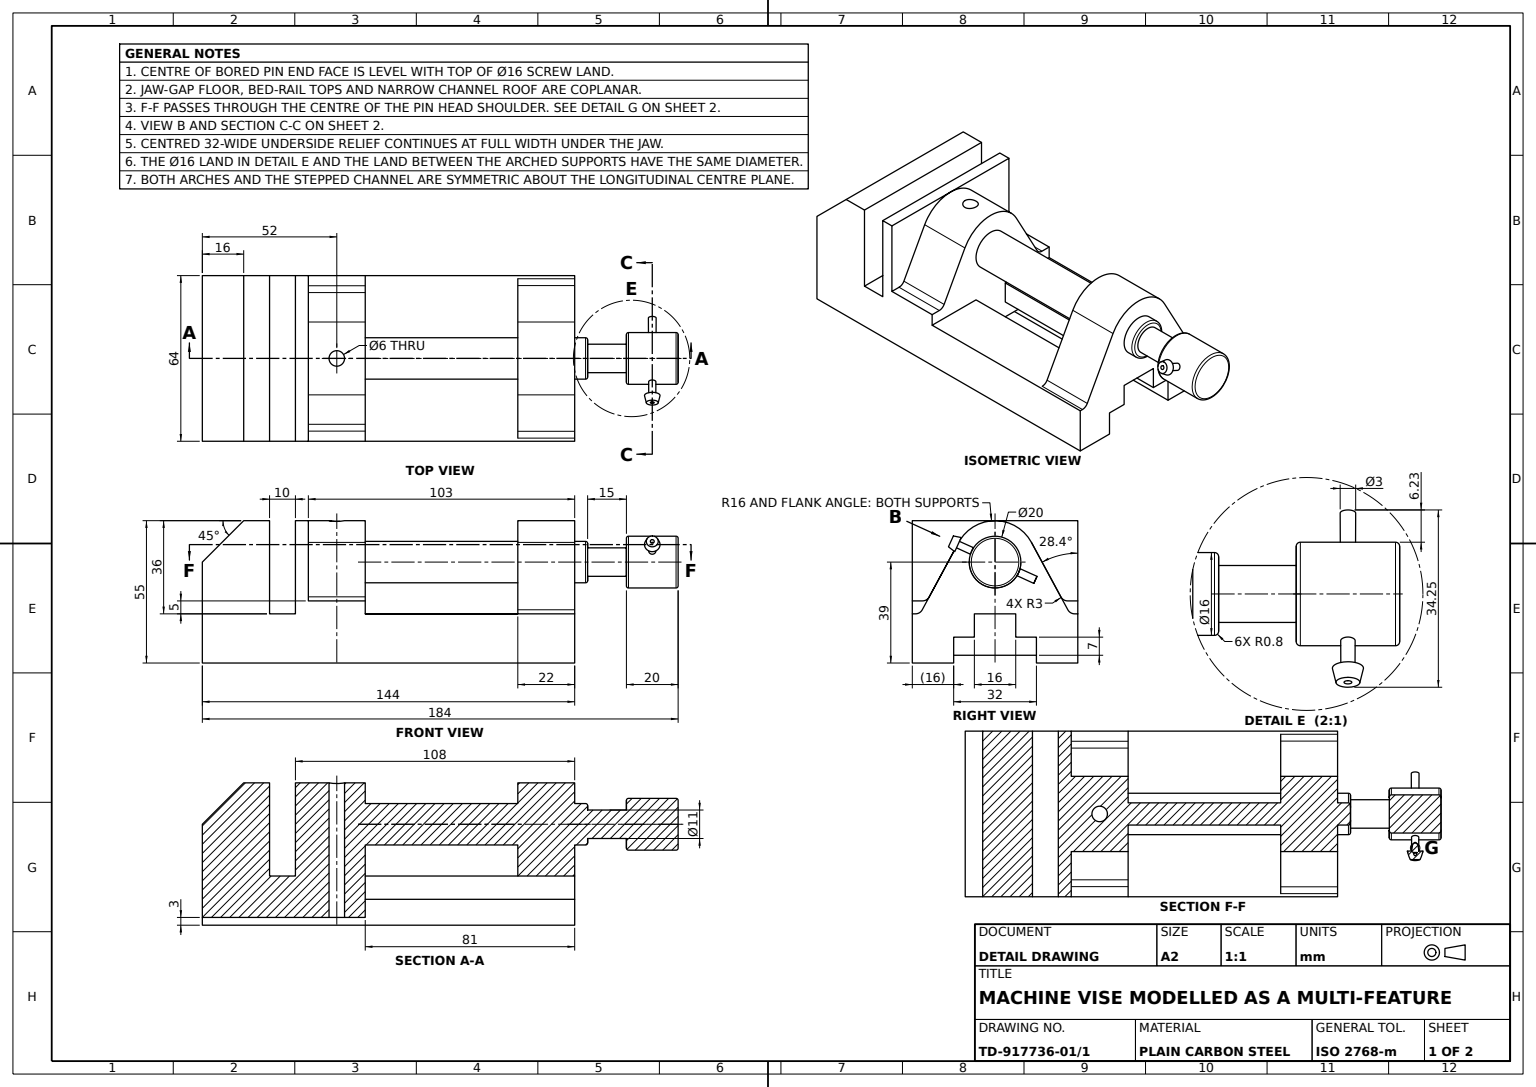
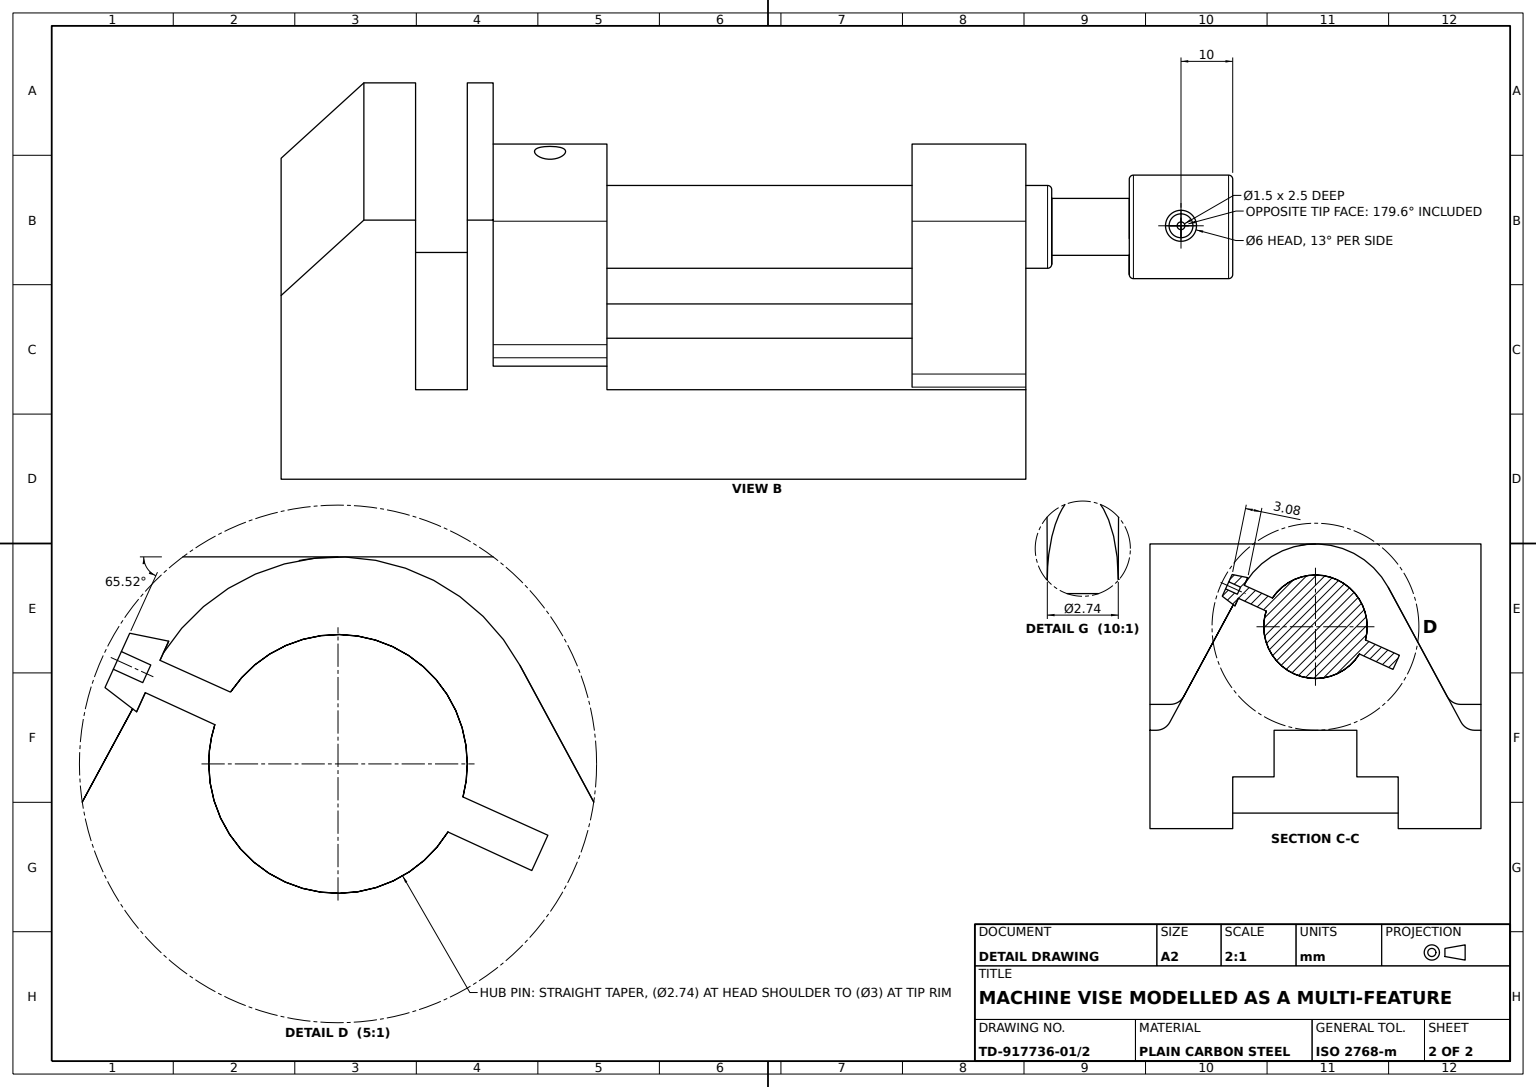
from build123d import *

# Parameters (mm, degrees)
VISE_BODY_DEPTH                 = 64
GUIDE_CHANNEL_PROFILE_OUTSIDE_W = 99.188
GUIDE_CHANNEL_PROFILE_OUTSIDE_H = 87.188
GUIDE_CHANNEL_CUT_DEPTH         = 81
SUPPORT_PLATE_PROFILE_W         = 64
SUPPORT_PLATE_PROFILE_H         = 52
SUPPORT_PLATE_DEPTH             = 5
JAW_START                       = 22
JAW_BLOCK_DEPTH                 = 22
LEAD_SCREW_SHAFT_16_DEPTH       = 5
LEAD_SCREW_SHAFT_16_DEPTH_BACK  = 81
LEAD_SCREW_PROFILE_16_R         = 8
SCREW_NECK_PROFILE_11_R         = 5.5
SCREW_NECK_11_DEPTH             = 15
HANDLE_HUB_PROFILE_20_R         = 10
HANDLE_HUB_20_DEPTH             = 20
JAW_BLOCK_FILLET_R3_R           = 3
JAW_BLOCK_CHANNEL_FILLET_R3_R   = 3
PIN_BOSS_PROFILE_6_R            = 3
PIN_BOSS_6_DEPTH                = 3
PIN_BOSS_6_TAPER                = 13
PIN_HOLE_PROFILE_1_5_R          = 0.75
PIN_HOLE_1_5_DEPTH              = 2.5
BASE_FOOT_PROFILE_W             = 144
BASE_FOOT_PROFILE_H             = 3
BASE_FOOT_DEPTH                 = 16
FOOT_EXTENSION_PROFILE_W        = 144
FOOT_EXTENSION_PROFILE_H        = 3
FOOT_EXTENSION_DEPTH            = 16
JAW_HOLE_PROFILE_6_R            = 3
JAW_HOLE_6_DEPTH                = 66
HANDLE_HUB_FILLET_R0_8_R        = 0.8
LEAD_SCREW_FILLET_R0_8_R        = 0.8


with BuildPart() as part:
    # Vise Body Profile → Vise Body (new body)
    with BuildSketch(Plane.XY):
        Polygon((0, 0), (0, 36), (16, 52), (26, 52), (26, 16), (122, 16), (122, 52), (144, 52), (144, 0), align=None)
    extrude(amount=VISE_BODY_DEPTH)

    # Guide Channel Profile outside → Guide Channel Cut (cut)
    with BuildSketch(Plane(origin=(144, 0, 0), x_dir=(0, 0, -1), z_dir=(1, 0, 0))):
        with Locations((-32, 26)):
            Rectangle(GUIDE_CHANNEL_PROFILE_OUTSIDE_W, GUIDE_CHANNEL_PROFILE_OUTSIDE_H)
        with BuildLine():
            Line((-64, 0), (-48, 0))
            Line((-48, 0), (-48, 7))
            Line((-48, 7), (-40, 7))
            Line((-40, 7), (-40, 16))
            Line((-40, 16), (-24, 16))
            Line((-24, 16), (-24, 7))
            Line((-24, 7), (-16, 7))
            Line((-16, 7), (-16, 0))
            Line((-16, 0), (0, 0))
            Line((0, 0), (0, 16))
            Line((0, 16), (-3, 16))
            Line((-3, 16), (-17.924974143, 43.608787493))
            ThreePointArc((-17.924974143, 43.608787493), (-32, 52), (-46.075025857, 43.608787493))
            Line((-46.075025857, 43.608787493), (-61, 16))
            Line((-61, 16), (-64, 16))
            Line((-64, 16), (-64, 0))
        make_face(mode=Mode.SUBTRACT)
    extrude(amount=-GUIDE_CHANNEL_CUT_DEPTH, mode=Mode.SUBTRACT)

    # Support Plate Profile → Support Plate (add)
    with BuildSketch(Plane(origin=(36, 0, 0), x_dir=(0, 0, -1), z_dir=(1, 0, 0))):
        with Locations((-32, 26)):
            Rectangle(SUPPORT_PLATE_PROFILE_W, SUPPORT_PLATE_PROFILE_H)
    extrude(amount=SUPPORT_PLATE_DEPTH)

    # Jaw Block Profile → Jaw Block (add)
    with BuildSketch(Plane(origin=(41, 0, 0), x_dir=(0, 0, -1), z_dir=(1, 0, 0)).offset(JAW_START)):
        with BuildLine():
            Line((-46.075025857, 43.608787493), (-58.297060918, 21))
            Line((-58.297060918, 21), (-64, 21))
            Line((-64, 21), (-64, 16))
            Line((-64, 16), (0, 16))
            Line((0, 16), (0, 21))
            Line((0, 21), (-5.702939082, 21))
            Line((-5.702939082, 21), (-17.924974143, 43.608787493))
            ThreePointArc((-17.924974143, 43.608787493), (-32, 52), (-46.075025857, 43.608787493))
        make_face()
    extrude(amount=-JAW_BLOCK_DEPTH)

    # Lead Screw Profile Ø16 → Lead Screw Shaft Ø16 (add, two sides: drawn at the far end of the back side and taken through both)
    with BuildSketch(Plane(origin=(144, 0, 0), x_dir=(0, 0, -1), z_dir=(1, 0, 0)).offset(-LEAD_SCREW_SHAFT_16_DEPTH_BACK)):
        with Locations((-32, 36)):
            Circle(LEAD_SCREW_PROFILE_16_R)
    extrude(amount=LEAD_SCREW_SHAFT_16_DEPTH + LEAD_SCREW_SHAFT_16_DEPTH_BACK)

    # Screw Neck Profile Ø11 → Screw Neck Ø11 (add)
    with BuildSketch(Plane(origin=(149, 0, 0), x_dir=(0, 0, -1), z_dir=(1, 0, 0))):
        with Locations((-32, 36)):
            Circle(SCREW_NECK_PROFILE_11_R)
    extrude(amount=SCREW_NECK_11_DEPTH)

    # Handle Hub Profile Ø20 → Handle Hub Ø20 (add)
    with BuildSketch(Plane(origin=(164, 0, 0), x_dir=(0, 0, -1), z_dir=(1, 0, 0))):
        with Locations((-32, 36)):
            Circle(HANDLE_HUB_PROFILE_20_R)
    extrude(amount=HANDLE_HUB_20_DEPTH)

    # Jaw Block Fillet R3
    jaw_block_fillet_r3_edges = [part.edges().sort_by_distance(p)[0] for p in [
        (52, 21, 58.297060918),
    ]]
    fillet(jaw_block_fillet_r3_edges, radius=JAW_BLOCK_FILLET_R3_R)

    # Jaw Block Channel Fillet R3
    jaw_block_channel_fillet_r3_edges = [part.edges().sort_by_distance(p)[0] for p in [
        (52, 21, 5.702939082),
        (133, 16, 3),
        (133, 16, 61),
    ]]
    fillet(jaw_block_channel_fillet_r3_edges, radius=JAW_BLOCK_CHANNEL_FILLET_R3_R)

    # Collar Revolve Profile → Collar Revolve (revolve)
    with BuildSketch(Plane(origin=(174, 0, 0), x_dir=(0, 0, -1), z_dir=(1, 0, 0)), mode=Mode.PRIVATE) as collar_revolve_sk:
        Polygon((-45.767721385, 44.00403367), (-15.767721385, 30.48840867), (-16.383860693, 29.120793097), (-46.336140932, 42.755332802), align=None)
    revolve(collar_revolve_sk.sketch.rotate(Axis((174, 47.778525514, 57.371062468), (0, -0.41430319244059016, -0.9101389260621344)), 209.202366006), axis=Axis((174, 47.778525514, 57.371062468), (0, -0.41430319244059016, -0.9101389260621344)))

    # Pin Boss Profile Ø6 → Pin Boss Ø6 (add)
    with BuildSketch(Plane(origin=(0, 24.810959499, 54.504576467), x_dir=(1, 0, 0), z_dir=(0, 0.41430319244059144, 0.9101389260621338))):
        with Locations((174, 19.716081566)):
            Circle(PIN_BOSS_PROFILE_6_R)
    extrude(amount=PIN_BOSS_6_DEPTH, taper=PIN_BOSS_6_TAPER)

    # Pin Hole Profile Ø1.5 → Pin Hole Ø1.5 (cut)
    with BuildSketch(Plane(origin=(0, 26.053869076, 57.234993245), x_dir=(1, 0, 0), z_dir=(0, 0.41430319244059144, 0.9101389260621339))):
        with Locations(Location((174, 19.716081566, 0), (0, 0, 270))):
            Circle(PIN_HOLE_PROFILE_1_5_R)
    extrude(amount=-PIN_HOLE_1_5_DEPTH, mode=Mode.SUBTRACT)

    # Base Foot Profile → Base Foot (add)
    with BuildSketch(Plane.XY.offset(64)):
        with Locations((72, -1.5)):
            Rectangle(BASE_FOOT_PROFILE_W, BASE_FOOT_PROFILE_H)
    extrude(amount=-BASE_FOOT_DEPTH)

    # Foot Extension Profile → Foot Extension (add)
    with BuildSketch(Plane(origin=(0, 0, 0), x_dir=(-1, 0, 0), z_dir=(0, 0, -1))):
        with Locations((-72, -1.5)):
            Rectangle(FOOT_EXTENSION_PROFILE_W, FOOT_EXTENSION_PROFILE_H)
    extrude(amount=-FOOT_EXTENSION_DEPTH)

    # Jaw Hole Profile Ø6 → Jaw Hole Ø6 (cut)
    with BuildSketch(Plane.XZ):
        with Locations((52, 32)):
            Circle(JAW_HOLE_PROFILE_6_R)
    extrude(amount=-JAW_HOLE_6_DEPTH, mode=Mode.SUBTRACT)

    # Handle Hub Fillet R0.8
    handle_hub_fillet_r0_8_edges = [part.edges().sort_by_distance(p)[0] for p in [
        (164, 36, 42),
        (184, 36, 42),
    ]]
    fillet(handle_hub_fillet_r0_8_edges, radius=HANDLE_HUB_FILLET_R0_8_R)

    # Lead Screw Fillet R0.8
    lead_screw_fillet_r0_8_edges = [part.edges().sort_by_distance(p)[0] for p in [
        (149, 36, 40),
    ]]
    fillet(lead_screw_fillet_r0_8_edges, radius=LEAD_SCREW_FILLET_R0_8_R)


solid = part.part
